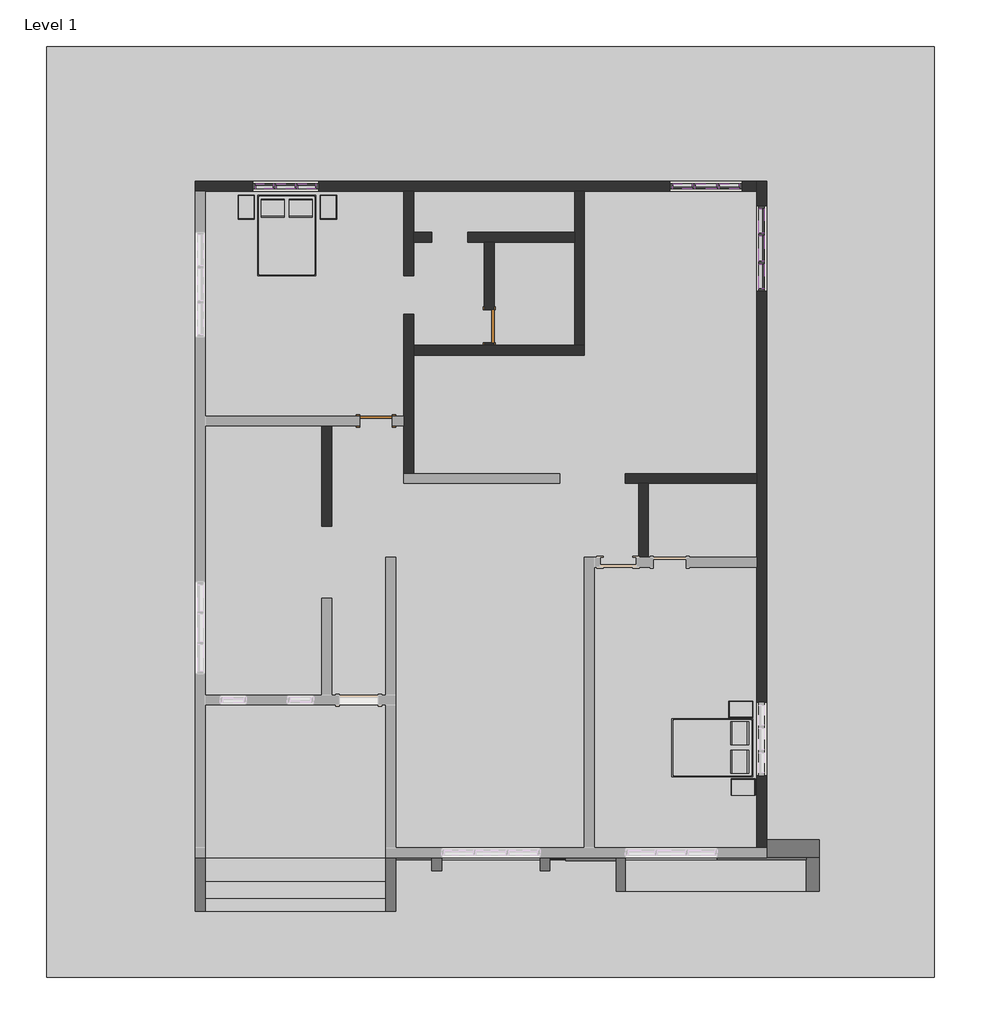
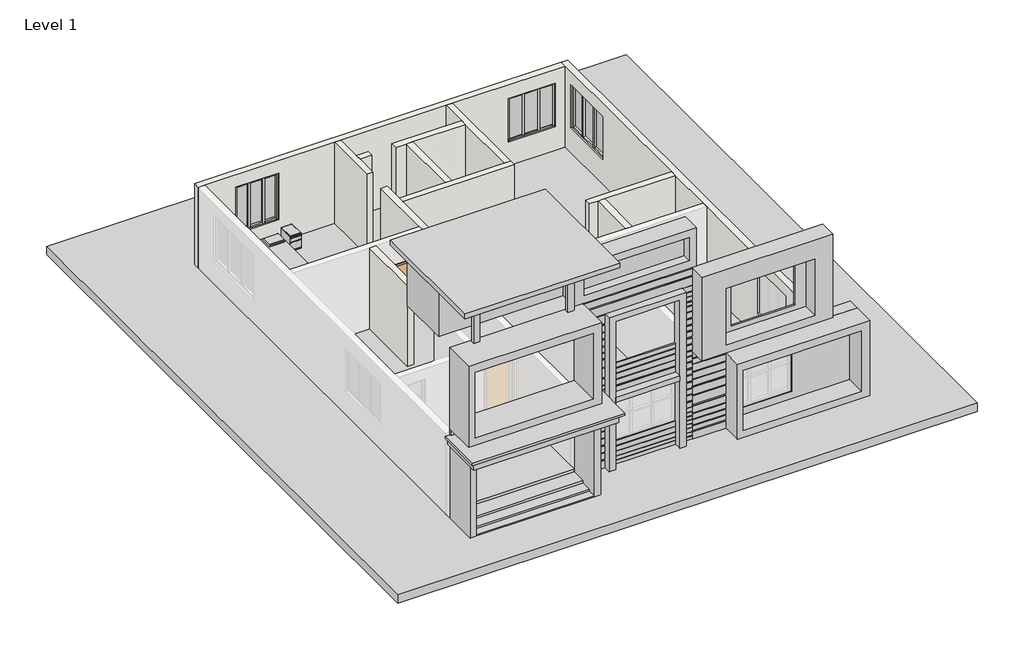
# One storey, part 3 of 3: 30 members, 12 walls, 9 plates, 6 furniture elements, 4 proxies, 2 doors.
"""IFC4 building model written with IfcOpenShell, lengths in millimetres."""

from ifc_helpers import new_model, si_unit, frame, origin, origin_with_axes, place, context, project, spatial, polyline, outline, extrude, faceted_brep, transform, mapped, element, save
from components import generic_models_1_generic_models_1_93a2076a, generic_models_2_generic_models_2_d251e182, generic_models_3_generic_models_3_e29e7d65, generic_models_4_generic_models_4_71b53b29, door_a1484949, furniture_b58f7881, furniture_b20b6c06, member_6f432376, member_a400357f, member_b7ff1776, member_d1d39edc, member_2ebf4a73, member_5535eeb3, member_ee21581d, member_a798bde5, member_dc106669, member_bc7dbe04, member_dded4e1f, member_1bc4b407, system_panel_glazed_a47e91a8, system_panel_glazed_a2afa025, system_panel_glazed_ca6a4ba2, system_panel_glazed_a9878b85, system_panel_glazed_435c231b, system_panel_glazed_676e31df

model = new_model("IFC4")

# Units and contexts
model_context = context("Model", 3, world=origin())
ifc_project = project(units=[si_unit("LENGTHUNIT", "METRE", prefix="MILLI")], contexts=[model_context])

# Site, building, storey
site = spatial("IfcSite", under=ifc_project)
building = spatial("IfcBuilding", under=site)
storey = spatial("IfcBuildingStorey", under=building, Name="Level 1", Elevation=0.0)

# Proxies
placement = place(None, origin())
generic_models_1_generic_models_1_shape = generic_models_1_generic_models_1_93a2076a(model_context)
element("IfcBuildingElementProxy", 1, Name="Generic Models 1 : Generic Models 1", ObjectType="Generic Models 1 : Generic Models 1", at=placement, inside=storey, context=model_context, shape_type="MappedRepresentation", body=[
    mapped(generic_models_1_generic_models_1_shape, transform((0.0, 0.0, 0.0), x_axis=(1.0, 0.0, 0.0), y_axis=(0.0, 1.0, 0.0), z_axis=(0.0, 0.0, 1.0))),
])
generic_models_2_generic_models_2_shape = generic_models_2_generic_models_2_d251e182(model_context)
element("IfcBuildingElementProxy", 2, Name="Generic Models 2 : Generic Models 2", ObjectType="Generic Models 2 : Generic Models 2", at=placement, inside=storey, context=model_context, shape_type="MappedRepresentation", body=[
    mapped(generic_models_2_generic_models_2_shape, transform((0.0, 0.0, 0.0), x_axis=(1.0, 0.0, 0.0), y_axis=(0.0, 1.0, 0.0), z_axis=(0.0, 0.0, 1.0))),
])
generic_models_3_generic_models_3_shape = generic_models_3_generic_models_3_e29e7d65(model_context)
element("IfcBuildingElementProxy", 3, Name="Generic Models 3 : Generic Models 3", ObjectType="Generic Models 3 : Generic Models 3", at=placement, inside=storey, context=model_context, shape_type="MappedRepresentation", body=[
    mapped(generic_models_3_generic_models_3_shape, transform((0.0, 0.0, 0.0), x_axis=(1.0, 0.0, 0.0), y_axis=(0.0, 1.0, 0.0), z_axis=(0.0, 0.0, 1.0))),
])
generic_models_4_generic_models_4_shape = generic_models_4_generic_models_4_71b53b29(model_context)
element("IfcBuildingElementProxy", 4, Name="Generic Models 4 : Generic Models 4", ObjectType="Generic Models 4 : Generic Models 4", at=placement, inside=storey, context=model_context, shape_type="MappedRepresentation", body=[
    mapped(generic_models_4_generic_models_4_shape, transform((0.0, 0.0, 0.0), x_axis=(1.0, 0.0, 0.0), y_axis=(0.0, 1.0, 0.0), z_axis=(0.0, 0.0, 1.0))),
])

# Doors
door_shape = door_a1484949(model_context)
element("IfcDoor", 5, ObjectType="Single-Flush : 30\" x 80\"", at=placement, inside=storey, context=model_context, shape_type="MappedRepresentation", body=[
    mapped(door_shape, transform((-14609.9127168, -4725.546149, 0.0), x_axis=(1.0, 0.0, 0.0), y_axis=(0.0, 1.0, 0.0), z_axis=(0.0, 0.0, 1.0))),
])
element("IfcDoor", 6, ObjectType="Single-Flush : 30\" x 80\"", at=placement, inside=storey, context=model_context, shape_type="MappedRepresentation", body=[
    mapped(door_shape, transform((-11980.7944131, -2528.446149, 0.0), x_axis=(0.0, -1.0, 0.0), y_axis=(1.0, 0.0, 0.0), z_axis=(0.0, 0.0, 1.0))),
])

# Furniture
furniture_shape = furniture_b58f7881(model_context)
element("IfcFurniture", 7, ObjectType="Bed-Box : Double 53\" x 74\"", at=placement, inside=storey, context=model_context, shape_type="MappedRepresentation", body=[
    mapped(furniture_shape, transform((-17019.1651758, -185.8166408, 0.0), x_axis=(1.0, 0.0, 0.0), y_axis=(0.0, 1.0, 0.0), z_axis=(0.0, 0.0, 1.0))),
])
element("IfcFurniture", 8, ObjectType="Bed-Box : Double 53\" x 74\"", at=placement, inside=storey, context=model_context, shape_type="MappedRepresentation", body=[
    mapped(furniture_shape, transform((-6564.5466012, -11968.29369, 0.0), x_axis=(0.0, -1.0, 0.0), y_axis=(1.0, 0.0, 0.0), z_axis=(0.0, 0.0, 1.0))),
])
furniture_2_shape = furniture_b20b6c06(model_context)
element("IfcFurniture", 9, ObjectType="Furniture_System-Storage-Cabinet-2_Drawer : 15\" x 22\" x 21\"", at=placement, inside=storey, context=model_context, shape_type="MappedRepresentation", body=[
    mapped(furniture_2_shape, transform((-15714.8127168, -39.246149, 0.0), x_axis=(1.0, 0.0, 0.0), y_axis=(0.0, 1.0, 0.0), z_axis=(0.0, 0.0, 1.0))),
])
element("IfcFurniture", 10, ObjectType="Furniture_System-Storage-Cabinet-2_Drawer : 15\" x 22\" x 21\"", at=placement, inside=storey, context=model_context, shape_type="MappedRepresentation", body=[
    mapped(furniture_2_shape, transform((-17619.8127168, -39.246149, 0.0), x_axis=(1.0, 0.0, 0.0), y_axis=(0.0, 1.0, 0.0), z_axis=(0.0, 0.0, 1.0))),
])
element("IfcFurniture", 11, ObjectType="Furniture_System-Storage-Cabinet-2_Drawer : 15\" x 22\" x 21\"", at=placement, inside=storey, context=model_context, shape_type="MappedRepresentation", body=[
    mapped(furniture_2_shape, transform((-6417.9761094, -11418.446149, 0.0), x_axis=(0.0, -1.0, 0.0), y_axis=(1.0, 0.0, 0.0), z_axis=(0.0, 0.0, 1.0))),
])
element("IfcFurniture", 12, ObjectType="Furniture_System-Storage-Cabinet-2_Drawer : 15\" x 22\" x 21\"", at=placement, inside=storey, context=model_context, shape_type="MappedRepresentation", body=[
    mapped(furniture_2_shape, transform((-6367.1761094, -13221.846149, 0.0), x_axis=(0.0, -1.0, 0.0), y_axis=(1.0, 0.0, 0.0), z_axis=(0.0, 0.0, 1.0))),
])

# Members
member_shape = member_6f432376(model_context)
element("IfcMember", 13, ObjectType="Rectangular Mullion : 2.5\" x 5\" rectangular", at=placement, inside=storey, context=model_context, shape_type="MappedRepresentation", body=[
    mapped(member_shape, transform((-5655.9761094, -363.096149, 2561.3470607), x_axis=(0.0, 0.0, 1.0), y_axis=(-1.0, 0.0, 0.0), z_axis=(0.0, -1.0, 0.0))),
])
element("IfcMember", 14, ObjectType="Rectangular Mullion : 2.5\" x 5\" rectangular", at=placement, inside=storey, context=model_context, shape_type="MappedRepresentation", body=[
    mapped(member_shape, transform((-5655.9761094, -1652.146149, 2561.3470607), x_axis=(0.0, 0.0, 1.0), y_axis=(-1.0, 0.0, 0.0), z_axis=(0.0, -1.0, 0.0))),
])
member_2_shape = member_a400357f(model_context)
element("IfcMember", 15, ObjectType="Rectangular Mullion : 2.5\" x 5\" rectangular", at=placement, inside=storey, context=model_context, shape_type="MappedRepresentation", body=[
    mapped(member_2_shape, transform((-5655.9761094, -1023.496149, 2561.3470607), x_axis=(0.0, 0.0, 1.0), y_axis=(-1.0, 0.0, 0.0), z_axis=(0.0, -1.0, 0.0))),
])
member_3_shape = member_b7ff1776(model_context)
element("IfcMember", 16, ObjectType="Rectangular Mullion : 2.5\" x 5\" rectangular", at=placement, inside=storey, context=model_context, shape_type="MappedRepresentation", body=[
    mapped(member_3_shape, transform((-5655.9761094, -394.846149, 937.2368213), x_axis=(0.0, -1.0, 0.0), y_axis=(-1.0, 0.0, 0.0), z_axis=(0.0, 0.0, -1.0))),
])
element("IfcMember", 17, ObjectType="Rectangular Mullion : 2.5\" x 5\" rectangular", at=placement, inside=storey, context=model_context, shape_type="MappedRepresentation", body=[
    mapped(member_3_shape, transform((-5655.9761094, -1055.246149, 937.2368213), x_axis=(0.0, -1.0, 0.0), y_axis=(-1.0, 0.0, 0.0), z_axis=(0.0, 0.0, -1.0))),
])
element("IfcMember", 18, ObjectType="Rectangular Mullion : 2.5\" x 5\" rectangular", at=placement, inside=storey, context=model_context, shape_type="MappedRepresentation", body=[
    mapped(member_2_shape, transform((-5655.9761094, -426.596149, 937.2368213), x_axis=(0.0, 0.0, -1.0), y_axis=(-1.0, 0.0, 0.0), z_axis=(0.0, 1.0, 0.0))),
])
element("IfcMember", 19, ObjectType="Rectangular Mullion : 2.5\" x 5\" rectangular", at=placement, inside=storey, context=model_context, shape_type="MappedRepresentation", body=[
    mapped(member_shape, transform((-5655.9761094, -1086.996149, 937.2368213), x_axis=(0.0, 0.0, -1.0), y_axis=(-1.0, 0.0, 0.0), z_axis=(0.0, 1.0, 0.0))),
])
element("IfcMember", 20, ObjectType="Rectangular Mullion : 2.5\" x 5\" rectangular", at=placement, inside=storey, context=model_context, shape_type="MappedRepresentation", body=[
    mapped(member_shape, transform((-5655.9761094, 202.053851, 937.2368213), x_axis=(0.0, 0.0, -1.0), y_axis=(-1.0, 0.0, 0.0), z_axis=(0.0, 1.0, 0.0))),
])
member_4_shape = member_d1d39edc(model_context)
element("IfcMember", 21, ObjectType="Rectangular Mullion : 2.5\" x 5\" rectangular", at=placement, inside=storey, context=model_context, shape_type="MappedRepresentation", body=[
    mapped(member_4_shape, transform((-5655.9761094, 265.553851, 2561.3470607), x_axis=(0.0, 1.0, 0.0), y_axis=(-1.0, 0.0, 0.0), z_axis=(0.0, 0.0, 1.0))),
])
element("IfcMember", 22, ObjectType="Rectangular Mullion : 2.5\" x 5\" rectangular", at=placement, inside=storey, context=model_context, shape_type="MappedRepresentation", body=[
    mapped(member_4_shape, transform((-5655.9761094, -1715.646149, 937.2368213), x_axis=(0.0, -1.0, 0.0), y_axis=(-1.0, 0.0, 0.0), z_axis=(0.0, 0.0, -1.0))),
])
member_5_shape = member_2ebf4a73(model_context)
element("IfcMember", 23, ObjectType="Rectangular Mullion : 2.5\" x 5\" rectangular", at=placement, inside=storey, context=model_context, shape_type="MappedRepresentation", body=[
    mapped(member_5_shape, transform((-7199.0261094, 722.753851, 2528.3677735), x_axis=(0.0, 0.0, 1.0), y_axis=(0.0, 1.0, 0.0), z_axis=(-1.0, 0.0, 0.0))),
])
member_6_shape = member_5535eeb3(model_context)
element("IfcMember", 24, ObjectType="Rectangular Mullion : 2.5\" x 5\" rectangular", at=placement, inside=storey, context=model_context, shape_type="MappedRepresentation", body=[
    mapped(member_6_shape, transform((-6640.2261094, 722.753851, 2528.3677735), x_axis=(0.0, 0.0, 1.0), y_axis=(0.0, 1.0, 0.0), z_axis=(-1.0, 0.0, 0.0))),
])
element("IfcMember", 25, ObjectType="Rectangular Mullion : 2.5\" x 5\" rectangular", at=placement, inside=storey, context=model_context, shape_type="MappedRepresentation", body=[
    mapped(member_6_shape, transform((-7726.0761094, 722.753851, 2528.3677735), x_axis=(0.0, 0.0, 1.0), y_axis=(0.0, 1.0, 0.0), z_axis=(-1.0, 0.0, 0.0))),
])
member_7_shape = member_ee21581d(model_context)
element("IfcMember", 26, ObjectType="Rectangular Mullion : 2.5\" x 5\" rectangular", at=placement, inside=storey, context=model_context, shape_type="MappedRepresentation", body=[
    mapped(member_7_shape, transform((-6671.9761094, 722.753851, 897.4359445), x_axis=(-1.0, 0.0, 0.0), y_axis=(0.0, 1.0, 0.0), z_axis=(0.0, 0.0, -1.0))),
])
element("IfcMember", 27, ObjectType="Rectangular Mullion : 2.5\" x 5\" rectangular", at=placement, inside=storey, context=model_context, shape_type="MappedRepresentation", body=[
    mapped(member_7_shape, transform((-7230.7761094, 722.753851, 897.4359445), x_axis=(-1.0, 0.0, 0.0), y_axis=(0.0, 1.0, 0.0), z_axis=(0.0, 0.0, -1.0))),
])
element("IfcMember", 28, ObjectType="Rectangular Mullion : 2.5\" x 5\" rectangular", at=placement, inside=storey, context=model_context, shape_type="MappedRepresentation", body=[
    mapped(member_6_shape, transform((-7262.5261094, 722.753851, 897.4359445), x_axis=(0.0, 0.0, -1.0), y_axis=(0.0, 1.0, 0.0), z_axis=(1.0, 0.0, 0.0))),
])
element("IfcMember", 29, ObjectType="Rectangular Mullion : 2.5\" x 5\" rectangular", at=placement, inside=storey, context=model_context, shape_type="MappedRepresentation", body=[
    mapped(member_6_shape, transform((-6176.6761094, 722.753851, 897.4359445), x_axis=(0.0, 0.0, -1.0), y_axis=(0.0, 1.0, 0.0), z_axis=(1.0, 0.0, 0.0))),
])
element("IfcMember", 30, ObjectType="Rectangular Mullion : 2.5\" x 5\" rectangular", at=placement, inside=storey, context=model_context, shape_type="MappedRepresentation", body=[
    mapped(member_5_shape, transform((-6703.7261094, 722.753851, 897.4359445), x_axis=(0.0, 0.0, -1.0), y_axis=(0.0, 1.0, 0.0), z_axis=(1.0, 0.0, 0.0))),
])
member_8_shape = member_a798bde5(model_context)
element("IfcMember", 31, ObjectType="Rectangular Mullion : 2.5\" x 5\" rectangular", at=placement, inside=storey, context=model_context, shape_type="MappedRepresentation", body=[
    mapped(member_8_shape, transform((-7789.5761094, 722.753851, 897.4359445), x_axis=(-1.0, 0.0, 0.0), y_axis=(0.0, 1.0, 0.0), z_axis=(0.0, 0.0, -1.0))),
])
element("IfcMember", 32, ObjectType="Rectangular Mullion : 2.5\" x 5\" rectangular", at=placement, inside=storey, context=model_context, shape_type="MappedRepresentation", body=[
    mapped(member_8_shape, transform((-6113.1761094, 722.753851, 2528.3677735), x_axis=(1.0, 0.0, 0.0), y_axis=(0.0, 1.0, 0.0), z_axis=(0.0, 0.0, 1.0))),
])
member_9_shape = member_dc106669(model_context)
element("IfcMember", 33, ObjectType="Rectangular Mullion : 2.5\" x 5\" rectangular", at=placement, inside=storey, context=model_context, shape_type="MappedRepresentation", body=[
    mapped(member_9_shape, transform((-16990.7261094, 722.753851, 2583.598837), x_axis=(0.0, 0.0, 1.0), y_axis=(0.0, -1.0, 0.0), z_axis=(1.0, 0.0, 0.0))),
])
element("IfcMember", 34, ObjectType="Rectangular Mullion : 2.5\" x 5\" rectangular", at=placement, inside=storey, context=model_context, shape_type="MappedRepresentation", body=[
    mapped(member_9_shape, transform((-16006.4761094, 722.753851, 2583.598837), x_axis=(0.0, 0.0, 1.0), y_axis=(0.0, -1.0, 0.0), z_axis=(1.0, 0.0, 0.0))),
])
member_10_shape = member_bc7dbe04(model_context)
element("IfcMember", 35, ObjectType="Rectangular Mullion : 2.5\" x 5\" rectangular", at=placement, inside=storey, context=model_context, shape_type="MappedRepresentation", body=[
    mapped(member_10_shape, transform((-16482.7261094, 722.753851, 2583.598837), x_axis=(0.0, 0.0, 1.0), y_axis=(0.0, -1.0, 0.0), z_axis=(1.0, 0.0, 0.0))),
])
member_11_shape = member_dded4e1f(model_context)
element("IfcMember", 36, ObjectType="Rectangular Mullion : 2.5\" x 5\" rectangular", at=placement, inside=storey, context=model_context, shape_type="MappedRepresentation", body=[
    mapped(member_11_shape, transform((-16450.9761094, 722.753851, 833.2365736), x_axis=(1.0, 0.0, 0.0), y_axis=(0.0, -1.0, 0.0), z_axis=(0.0, 0.0, -1.0))),
])
element("IfcMember", 37, ObjectType="Rectangular Mullion : 2.5\" x 5\" rectangular", at=placement, inside=storey, context=model_context, shape_type="MappedRepresentation", body=[
    mapped(member_11_shape, transform((-16958.9761094, 722.753851, 833.2365736), x_axis=(1.0, 0.0, 0.0), y_axis=(0.0, -1.0, 0.0), z_axis=(0.0, 0.0, -1.0))),
])
element("IfcMember", 38, ObjectType="Rectangular Mullion : 2.5\" x 5\" rectangular", at=placement, inside=storey, context=model_context, shape_type="MappedRepresentation", body=[
    mapped(member_10_shape, transform((-16927.2261094, 722.753851, 833.2365736), x_axis=(0.0, 0.0, -1.0), y_axis=(0.0, -1.0, 0.0), z_axis=(-1.0, 0.0, 0.0))),
])
element("IfcMember", 39, ObjectType="Rectangular Mullion : 2.5\" x 5\" rectangular", at=placement, inside=storey, context=model_context, shape_type="MappedRepresentation", body=[
    mapped(member_9_shape, transform((-16419.2261094, 722.753851, 833.2365736), x_axis=(0.0, 0.0, -1.0), y_axis=(0.0, -1.0, 0.0), z_axis=(-1.0, 0.0, 0.0))),
])
element("IfcMember", 40, ObjectType="Rectangular Mullion : 2.5\" x 5\" rectangular", at=placement, inside=storey, context=model_context, shape_type="MappedRepresentation", body=[
    mapped(member_9_shape, transform((-17403.4761094, 722.753851, 833.2365736), x_axis=(0.0, 0.0, -1.0), y_axis=(0.0, -1.0, 0.0), z_axis=(-1.0, 0.0, 0.0))),
])
member_12_shape = member_1bc4b407(model_context)
element("IfcMember", 41, ObjectType="Rectangular Mullion : 2.5\" x 5\" rectangular", at=placement, inside=storey, context=model_context, shape_type="MappedRepresentation", body=[
    mapped(member_12_shape, transform((-15942.9761094, 722.753851, 833.2365736), x_axis=(1.0, 0.0, 0.0), y_axis=(0.0, -1.0, 0.0), z_axis=(0.0, 0.0, -1.0))),
])
element("IfcMember", 42, ObjectType="Rectangular Mullion : 2.5\" x 5\" rectangular", at=placement, inside=storey, context=model_context, shape_type="MappedRepresentation", body=[
    mapped(member_12_shape, transform((-17466.9761094, 722.753851, 2583.598837), x_axis=(-1.0, 0.0, 0.0), y_axis=(0.0, -1.0, 0.0), z_axis=(0.0, 0.0, 1.0))),
])

# Plates
system_panel_glazed_shape = system_panel_glazed_a47e91a8(model_context)
element("IfcPlate", 43, ObjectType="System Panel : Glazed", at=placement, inside=storey, context=model_context, shape_type="MappedRepresentation", body=[
    mapped(system_panel_glazed_shape, transform((-5655.9761094, -80.521149, 1000.7368213), x_axis=(0.0, -1.0, 0.0), y_axis=(1.0, 0.0, 0.0), z_axis=(0.0, 0.0, 1.0))),
])
element("IfcPlate", 44, ObjectType="System Panel : Glazed", at=placement, inside=storey, context=model_context, shape_type="MappedRepresentation", body=[
    mapped(system_panel_glazed_shape, transform((-5655.9761094, -1369.571149, 1000.7368213), x_axis=(0.0, -1.0, 0.0), y_axis=(1.0, 0.0, 0.0), z_axis=(0.0, 0.0, 1.0))),
])
system_panel_glazed_2_shape = system_panel_glazed_a2afa025(model_context)
element("IfcPlate", 45, ObjectType="System Panel : Glazed", at=placement, inside=storey, context=model_context, shape_type="MappedRepresentation", body=[
    mapped(system_panel_glazed_2_shape, transform((-5655.9761094, -725.046149, 1000.7368213), x_axis=(0.0, -1.0, 0.0), y_axis=(1.0, 0.0, 0.0), z_axis=(0.0, 0.0, 1.0))),
])
system_panel_glazed_3_shape = system_panel_glazed_ca6a4ba2(model_context)
element("IfcPlate", 46, ObjectType="System Panel : Glazed", at=placement, inside=storey, context=model_context, shape_type="MappedRepresentation", body=[
    mapped(system_panel_glazed_3_shape, transform((-6408.4511094, 722.753851, 960.9359445), x_axis=(-1.0, 0.0, 0.0), y_axis=(0.0, -1.0, 0.0), z_axis=(0.0, 0.0, 1.0))),
])
element("IfcPlate", 47, ObjectType="System Panel : Glazed", at=placement, inside=storey, context=model_context, shape_type="MappedRepresentation", body=[
    mapped(system_panel_glazed_3_shape, transform((-7494.3011094, 722.753851, 960.9359445), x_axis=(-1.0, 0.0, 0.0), y_axis=(0.0, -1.0, 0.0), z_axis=(0.0, 0.0, 1.0))),
])
system_panel_glazed_4_shape = system_panel_glazed_a9878b85(model_context)
element("IfcPlate", 48, ObjectType="System Panel : Glazed", at=placement, inside=storey, context=model_context, shape_type="MappedRepresentation", body=[
    mapped(system_panel_glazed_4_shape, transform((-6951.3761094, 722.753851, 960.9359445), x_axis=(-1.0, 0.0, 0.0), y_axis=(0.0, -1.0, 0.0), z_axis=(0.0, 0.0, 1.0))),
])
system_panel_glazed_5_shape = system_panel_glazed_435c231b(model_context)
element("IfcPlate", 49, ObjectType="System Panel : Glazed", at=placement, inside=storey, context=model_context, shape_type="MappedRepresentation", body=[
    mapped(system_panel_glazed_5_shape, transform((-17197.1011094, 722.753851, 896.7365736), x_axis=(1.0, 0.0, 0.0), y_axis=(0.0, 1.0, 0.0), z_axis=(0.0, 0.0, 1.0))),
])
element("IfcPlate", 50, ObjectType="System Panel : Glazed", at=placement, inside=storey, context=model_context, shape_type="MappedRepresentation", body=[
    mapped(system_panel_glazed_5_shape, transform((-16212.8511094, 722.753851, 896.7365736), x_axis=(1.0, 0.0, 0.0), y_axis=(0.0, 1.0, 0.0), z_axis=(0.0, 0.0, 1.0))),
])
system_panel_glazed_6_shape = system_panel_glazed_676e31df(model_context)
element("IfcPlate", 51, ObjectType="System Panel : Glazed", at=placement, inside=storey, context=model_context, shape_type="MappedRepresentation", body=[
    mapped(system_panel_glazed_6_shape, transform((-16704.9761094, 722.753851, 896.7365736), x_axis=(1.0, 0.0, 0.0), y_axis=(0.0, 1.0, 0.0), z_axis=(0.0, 0.0, 1.0))),
])

# Walls
element("IfcWall", 52, ObjectType="9\"", at=placement, inside=storey, context=model_context, shape_type="Brep", body=[
    faceted_brep([(-5541.6761094, -14631.546149, 0.0), (-5541.6761094, 837.053851, 0.0), (-5541.6761094, 837.053851, 3048.0), (-5541.6761094, -14631.546149, 3048.0), (-5541.6761094, -12958.2990397, 945.2248153), (-5541.6761094, -12958.2990397, 2620.512388), (-5541.6761094, -11256.4990397, 2620.512388), (-5541.6761094, -11256.4990397, 945.2248153), (-5541.6761094, 265.553851, 2561.3470607), (-5541.6761094, 265.553851, 937.2368213), (-5541.6761094, -1715.646149, 937.2368213), (-5541.6761094, -1715.646149, 2561.3470607), (-5770.2761094, 837.053851, 0.0), (-5770.2761094, 608.453851, 0.0), (-5770.2761094, -5944.746149, 0.0), (-5770.2761094, -6173.346149, 0.0), (-5770.2761094, -7887.846149, 0.0), (-5770.2761094, -8116.446149, 0.0), (-5770.2761094, -14631.546149, 0.0), (-5770.2761094, -14631.546149, 3048.0), (-5770.2761094, -8116.446149, 3048.0), (-5770.2761094, -7887.846149, 3048.0), (-5770.2761094, -6173.346149, 3048.0), (-5770.2761094, -5944.746149, 3048.0), (-5770.2761094, 608.453851, 3048.0), (-5770.2761094, 837.053851, 3048.0), (-5770.2761094, -12958.2990397, 2620.512388), (-5770.2761094, -12958.2990397, 945.2248153), (-5770.2761094, -11256.4990397, 945.2248153), (-5770.2761094, -11256.4990397, 2620.512388), (-5770.2761094, 265.553851, 937.2368213), (-5770.2761094, 265.553851, 2561.3470607), (-5770.2761094, -1715.646149, 2561.3470607), (-5770.2761094, -1715.646149, 937.2368213)], [[[0, 1, 2, 3], [4, 5, 6, 7], [8, 9, 10, 11]], [[12, 13, 14, 15, 16, 17, 18, 19, 20, 21, 22, 23, 24, 25], [26, 27, 28, 29], [30, 31, 32, 33]], [[1, 0, 18, 17, 16, 15, 14, 13, 12]], [[3, 2, 25, 24, 23, 22, 21, 20, 19]], [[0, 3, 19, 18]], [[2, 1, 12, 25]], [[26, 5, 4, 27]], [[5, 26, 29, 6]], [[6, 29, 28, 7]], [[27, 4, 7, 28]], [[30, 9, 8, 31]], [[31, 8, 11, 32]], [[32, 11, 10, 33]], [[9, 30, 33, 10]]]),
])
element("IfcWall", 53, ObjectType="9\"", at=placement, inside=storey, context=model_context, shape_type="Brep", body=[
    faceted_brep([(-5770.2761094, 837.053851, 0.0), (-18800.4761094, 837.053851, 0.0), (-18800.4761094, 837.053851, 3048.0), (-5770.2761094, 837.053851, 3048.0), (-6113.1761094, 837.053851, 897.4359445), (-6113.1761094, 837.053851, 2528.3677735), (-7789.5761094, 837.053851, 2528.3677735), (-7789.5761094, 837.053851, 897.4359445), (-17466.9761094, 837.053851, 2583.598837), (-17466.9761094, 837.053851, 833.2365736), (-15942.9761094, 837.053851, 833.2365736), (-15942.9761094, 837.053851, 2583.598837), (-18800.4761094, 608.453851, 0.0), (-18571.8761094, 608.453851, 0.0), (-13962.2127168, 608.453851, 0.0), (-13733.6127168, 608.453851, 0.0), (-9999.3761094, 608.453851, 0.0), (-9770.7761094, 608.453851, 0.0), (-5770.2761094, 608.453851, 0.0), (-5770.2761094, 608.453851, 3048.0), (-9770.7761094, 608.453851, 3048.0), (-9999.3761094, 608.453851, 3048.0), (-13733.6127168, 608.453851, 3048.0), (-13962.2127168, 608.453851, 3048.0), (-18571.8761094, 608.453851, 3048.0), (-18800.4761094, 608.453851, 3048.0), (-6113.1761094, 608.453851, 2528.3677735), (-6113.1761094, 608.453851, 897.4359445), (-7789.5761094, 608.453851, 897.4359445), (-7789.5761094, 608.453851, 2528.3677735), (-17466.9761094, 608.453851, 833.2365736), (-17466.9761094, 608.453851, 2583.598837), (-15942.9761094, 608.453851, 2583.598837), (-15942.9761094, 608.453851, 833.2365736)], [[[0, 1, 2, 3], [4, 5, 6, 7], [8, 9, 10, 11]], [[12, 13, 14, 15, 16, 17, 18, 19, 20, 21, 22, 23, 24, 25], [26, 27, 28, 29], [30, 31, 32, 33]], [[1, 0, 18, 17, 16, 15, 14, 13, 12]], [[3, 2, 25, 24, 23, 22, 21, 20, 19]], [[0, 3, 19, 18]], [[2, 1, 12, 25]], [[26, 5, 4, 27]], [[5, 26, 29, 6]], [[6, 29, 28, 7]], [[27, 4, 7, 28]], [[30, 9, 8, 31]], [[31, 8, 11, 32]], [[32, 11, 10, 33]], [[9, 30, 33, 10]]]),
])
element("IfcWall", 54, ObjectType="9\"", at=placement, inside=storey, context=model_context, shape_type="Brep", body=[
    faceted_brep([(-5770.2761094, -5944.746149, 0.0), (-8818.7127168, -5944.746149, 0.0), (-8818.7127168, -5944.746149, 3048.0), (-5770.2761094, -5944.746149, 3048.0), (-5770.2761094, -6173.346149, 0.0), (-5770.2761094, -6173.346149, 3048.0), (-8284.8761094, -6173.346149, 3048.0), (-8513.4761094, -6173.346149, 3048.0), (-8818.7127168, -6173.346149, 3048.0), (-8818.7127168, -6173.346149, 0.0), (-8513.4761094, -6173.346149, 0.0), (-8284.8761094, -6173.346149, 0.0)], [[[0, 1, 2, 3]], [[4, 5, 6, 7, 8, 9, 10, 11]], [[1, 0, 4, 11, 10, 9]], [[2, 1, 9, 8]], [[3, 2, 8, 7, 6, 5]], [[0, 3, 5, 4]]]),
])
element("IfcWall", 55, ObjectType="9\"", at=placement, inside=storey, context=model_context, shape_type="Brep", body=[
    faceted_brep([(-13733.6127168, -5944.746149, 0.0), (-13733.6127168, -3201.546149, 0.0), (-13733.6127168, -2972.946149, 0.0), (-13733.6127168, -2249.046149, 0.0), (-13733.6127168, -2249.046149, 3048.0), (-13733.6127168, -2972.946149, 3048.0), (-13733.6127168, -3201.546149, 3048.0), (-13733.6127168, -5944.746149, 3048.0), (-13962.2127168, -5944.746149, 0.0), (-13962.2127168, -5944.746149, 3048.0), (-13962.2127168, -4839.846149, 3048.0), (-13962.2127168, -4611.246149, 3048.0), (-13962.2127168, -2249.046149, 3048.0), (-13962.2127168, -2249.046149, 0.0), (-13962.2127168, -4611.246149, 0.0), (-13962.2127168, -4839.846149, 0.0)], [[[0, 1, 2, 3, 4, 5, 6, 7]], [[8, 9, 10, 11, 12, 13, 14, 15]], [[3, 2, 1, 0, 8, 15, 14, 13]], [[4, 3, 13, 12]], [[7, 6, 5, 4, 12, 11, 10, 9]], [[0, 7, 9, 8]]]),
])
element("IfcWall", 56, ObjectType="9\"", at=placement, inside=storey, context=model_context, shape_type="Brep", body=[
    faceted_brep([(-13733.6127168, -3201.546149, 0.0), (-9770.7761094, -3201.546149, 0.0), (-9770.7761094, -3201.546149, 3048.0), (-13733.6127168, -3201.546149, 3048.0), (-13733.6127168, -2972.946149, 0.0), (-13733.6127168, -2972.946149, 3048.0), (-12095.0944131, -2972.946149, 3048.0), (-11866.4944131, -2972.946149, 3048.0), (-9999.3761094, -2972.946149, 3048.0), (-9770.7761094, -2972.946149, 3048.0), (-9770.7761094, -2972.946149, 0.0), (-9999.3761094, -2972.946149, 0.0), (-11866.4944131, -2972.946149, 0.0), (-12095.0944131, -2972.946149, 0.0)], [[[0, 1, 2, 3]], [[4, 5, 6, 7, 8, 9, 10, 11, 12, 13]], [[1, 0, 4, 13, 12, 11, 10]], [[3, 2, 9, 8, 7, 6, 5]], [[0, 3, 5, 4]], [[2, 1, 10, 9]]]),
])
element("IfcWall", 57, ObjectType="9\"", at=placement, inside=storey, context=model_context, shape_type="Brep", body=[
    faceted_brep([(-9770.7761094, -2972.946149, 0.0), (-9770.7761094, 608.453851, 0.0), (-9770.7761094, 608.453851, 3048.0), (-9770.7761094, -2972.946149, 3048.0), (-9999.3761094, -2972.946149, 0.0), (-9999.3761094, -2972.946149, 3048.0), (-9999.3761094, -572.646149, 3048.0), (-9999.3761094, -344.046149, 3048.0), (-9999.3761094, 608.453851, 3048.0), (-9999.3761094, 608.453851, 0.0), (-9999.3761094, -344.046149, 0.0), (-9999.3761094, -572.646149, 0.0)], [[[0, 1, 2, 3]], [[4, 5, 6, 7, 8, 9, 10, 11]], [[1, 0, 4, 11, 10, 9]], [[3, 2, 8, 7, 6, 5]], [[0, 3, 5, 4]], [[2, 1, 9, 8]]]),
])
element("IfcWall", 58, ObjectType="9\"", at=placement, inside=storey, context=model_context, shape_type="SweptSolid", body=[
    extrude(outline(polyline([(-13314.5127168, -572.646149), (-13733.6127168, -572.646149), (-13733.6127168, -344.046149), (-13314.5127168, -344.046149), (-13314.5127168, -572.646149)])), origin_with_axes(), (0.0, 0.0, 1.0), 3048.0),
])
element("IfcWall", 59, ObjectType="9\"", at=placement, inside=storey, context=model_context, shape_type="SweptSolid", body=[
    extrude(outline(polyline([(-2909.446149, 2032.0), (-2909.446149, 0.0), (-2972.946149, 0.0), (-2972.946149, 3048.0), (-572.646149, 3048.0), (-572.646149, 0.0), (-2147.446149, 0.0), (-2147.446149, 2032.0), (-2909.446149, 2032.0)])), frame((-12095.0944131, 0.0, 0.0), z_axis=(1.0, 0.0, 0.0), x_axis=(0.0, 1.0, 0.0)), (0.0, 0.0, 1.0), 228.6),
])
element("IfcWall", 60, ObjectType="9\"", at=placement, inside=storey, context=model_context, shape_type="SweptSolid", body=[
    extrude(outline(polyline([(-15866.7761094, -7163.946149), (-15866.7761094, -4839.846149), (-15638.1761094, -4839.846149), (-15638.1761094, -7163.946149), (-15866.7761094, -7163.946149)])), origin_with_axes(), (0.0, 0.0, 1.0), 3048.0),
])
element("IfcWall", 61, ObjectType="9\"", at=placement, inside=storey, context=model_context, shape_type="SweptSolid", body=[
    extrude(outline(polyline([(-8513.4761094, -7887.846149), (-8513.4761094, -6173.346149), (-8284.8761094, -6173.346149), (-8284.8761094, -7887.846149), (-8513.4761094, -7887.846149)])), origin_with_axes(), (0.0, 0.0, 1.0), 3048.0),
])
element("IfcWall", 62, ObjectType="9\"", at=placement, inside=storey, context=model_context, shape_type="Brep", body=[
    faceted_brep([(-13733.6127168, -1360.046149, 0.0), (-13733.6127168, -572.646149, 0.0), (-13733.6127168, -344.046149, 0.0), (-13733.6127168, 608.453851, 0.0), (-13733.6127168, 608.453851, 3048.0), (-13733.6127168, -344.046149, 3048.0), (-13733.6127168, -572.646149, 3048.0), (-13733.6127168, -1360.046149, 3048.0), (-13962.2127168, -1360.046149, 0.0), (-13962.2127168, -1360.046149, 3048.0), (-13962.2127168, 608.453851, 3048.0), (-13962.2127168, 608.453851, 0.0)], [[[0, 1, 2, 3, 4, 5, 6, 7]], [[8, 9, 10, 11]], [[3, 2, 1, 0, 8, 11]], [[7, 6, 5, 4, 10, 9]], [[0, 7, 9, 8]], [[4, 3, 11, 10]]]),
])
element("IfcWall", 63, ObjectType="9\"", at=placement, inside=storey, context=model_context, shape_type="Brep", body=[
    faceted_brep([(-12476.3127168, -572.646149, 0.0), (-12095.0944131, -572.646149, 0.0), (-11866.4944131, -572.646149, 0.0), (-9999.3761094, -572.646149, 0.0), (-9999.3761094, -572.646149, 3048.0), (-11866.4944131, -572.646149, 3048.0), (-12095.0944131, -572.646149, 3048.0), (-12476.3127168, -572.646149, 3048.0), (-12476.3127168, -344.046149, 0.0), (-12476.3127168, -344.046149, 3048.0), (-9999.3761094, -344.046149, 3048.0), (-9999.3761094, -344.046149, 0.0)], [[[0, 1, 2, 3, 4, 5, 6, 7]], [[8, 9, 10, 11]], [[3, 2, 1, 0, 8, 11]], [[7, 6, 5, 4, 10, 9]], [[0, 7, 9, 8]], [[4, 3, 11, 10]]]),
])

save(model, "model.ifc")

# Revit data of these elements
# Type "Single-Flush : 30\" x 80\""
#   Type Mark = "5"
#   Construction Type Id = "MDOOR"
#   Assembly Code = "C1020"
#   Analytic Construction = "Metal"
#   Thickness = 0' - 2"
#   Heat Transfer Coefficient (U) = 0.651978 BTU/(h·ft²·°F)
#   Height = 6' - 8"
#   Trim Projection Ext = 0' - 1"
#   Trim Projection Int = 0' - 1"
#   Trim Width = 0' - 3"
#   Width = 2' - 6"
#   Define Thermal Properties by = 1
#   Define Thermal Properties by = 1
#   Door Material = Door - Panel
#   Frame Material = Door - Frame
#   Visual Light Transmittance = 0
#   Solar Heat Gain Coefficient = 0
#   Function = (empty or 0)
#   Wall Closure = (empty or 0)
# Type "Bed-Box : Double 53\" x 74\""
#   Assembly Code = "E2020200"
#   Length = 6' - 2"
#   Width = 4' - 5"
#   Frame Material = Birch
#   Mattress Material = Linen, White
#   Default Elevation = 0
# Type "Furniture_System-Storage-Cabinet-2_Drawer : 15\" x 22\" x 21\""
#   Type Comments = "15\" x 22\" x 21\" Double Drawer Cabinet"
#   Width = 1' - 3"
#   Height = 1' - 9"
#   Depth = 1' - 10"
#   Show Solid [instance default] = yes
#   Show Dashed [instance default] = no
#   Seat Visible [instance default] = yes
#   Drawer Material [instance default] = Metal - Paint - Beige
#   Cabinet Material [instance default] = Metal - Paint - Beige
#   Model = ""
#   Manufacturer = ""
#   Keynote = ""
#   Description = (empty or 0)
#   Default Elevation = 0
# Type "Rectangular Mullion : 2.5\" x 5\" rectangular"
#   built-in parameter 1007304 = 0.416667 (stored number, unit not read)
#   built-in parameter 1007301 = 0.104167 (stored number, unit not read)
#   built-in parameter 1007300 = 0.104167 (stored number, unit not read)
# Type "System Panel : Glazed"
#   Construction Type Id = "GSP4R"
#   Analytic Construction = "1/8 in Pilkington single glazing"
#   Visual Light Transmittance = 0.9
#   Solar Heat Gain Coefficient = 0.86
#   Heat Transfer Coefficient (U) = 1.18115 BTU/(h·ft²·°F)
#   Define Thermal Properties by = 1
# Type "9\""
#   Assembly Code = "B2010"
#   Layers, outside or top first: 0' - 9" no material (function 1)
# Element 1 (IfcBuildingElementProxy, "Generic Models 1 : Generic Models 1")
#   Phase Created = New Construction
# Element 2 (IfcBuildingElementProxy, "Generic Models 2 : Generic Models 2")
#   Phase Created = New Construction
# Element 3 (IfcBuildingElementProxy, "Generic Models 3 : Generic Models 3")
#   Phase Created = New Construction
# Element 4 (IfcBuildingElementProxy, "Generic Models 4 : Generic Models 4")
#   Phase Created = New Construction
# Elements 5, 6 (IfcDoor, "Single-Flush : 30\" x 80\"")
#   Phase Created = New Construction
#   Materials on its faces: "Door - Frame", "Door - Panel"
# Elements 7, 8 (IfcFurniture, "Bed-Box : Double 53\" x 74\"")
#   Phase Created = New Construction
#   Materials on its faces: "Birch", "Linen, White"
# Elements 9, 10, 11, 12 (IfcFurniture, "Furniture_System-Storage-Cabinet-2_Drawer : 15\" x 22\" x 21\"")
#   Show Solid = yes
#   Show Dashed = no
#   Seat Visible = yes
#   Drawer Material = Metal - Paint - Beige
#   Cabinet Material = Metal - Paint - Beige
#   Phase Created = New Construction
#   Materials on its faces: "Metal - Paint - Beige"
# Elements 13, 14, 15, 16, 17, 18, 19, 20, 21, 22, 23, 24, 25, 26, 27, 28, 29, 30, 31, 32, 33, 34, 35, 36, 37, 38, 39, 40, 41, 42 (IfcMember, "Rectangular Mullion : 2.5\" x 5\" rectangular")
#   Phase Created = New Construction
#   Materials on its faces: "Aluminum"
# Elements 43, 44, 45, 46, 47, 48, 49, 50, 51 (IfcPlate, "System Panel : Glazed")
#   Phase Created = New Construction
#   Materials on its faces: "Glass"
# Elements 52, 53, 54, 55, 56, 57, 58, 59, 60, 61, 62, 63 (IfcWall, "9\"")
#   Top Offset = 0' - 0"
#   Base Offset = 0' - 0"
#   Unconnected Height = 10' - 0"
#   wall height = 10' - 0"
#   Phase Created = New Construction
#   Base Constraint = Level 1
#   Materials on its faces: "Default Wall"
# Materials
#   "Door - Panel": class "Wood", colour RGB 210 159 95, transparency 0, Cost = 0
#   "Door - Frame": colour RGB 118 70 51, transparency 0, Cost = 0
#   "Birch": class "Wood", colour RGB 224 178 126, transparency 0, Description = "Betula Alleghaniensis", Cost = 0
#   "Linen, White": class "Textile", colour RGB 247 247 239, transparency 0, Description = "Linen, white", Cost = 0
#   "Metal - Paint - Beige": class "Metal", colour RGB 247 225 182, transparency 0
#   "Aluminum": class "Metal", colour RGB 247 247 247, transparency 0, Description = "Aluminum 6061", Cost = 0
#   "Glass": class "Glass", colour RGB 0 128 192, transparency 0.75, Description = "Soda Lime Glass", Cost = 0
#   "Default Wall": colour RGB 128 128 128, transparency 0, Cost = 0
